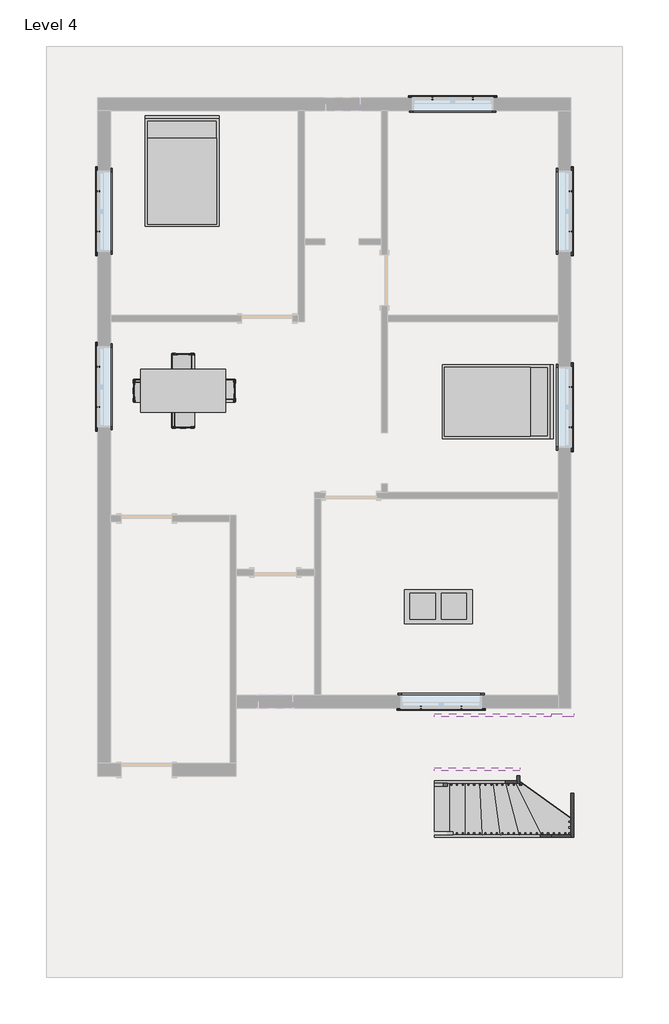
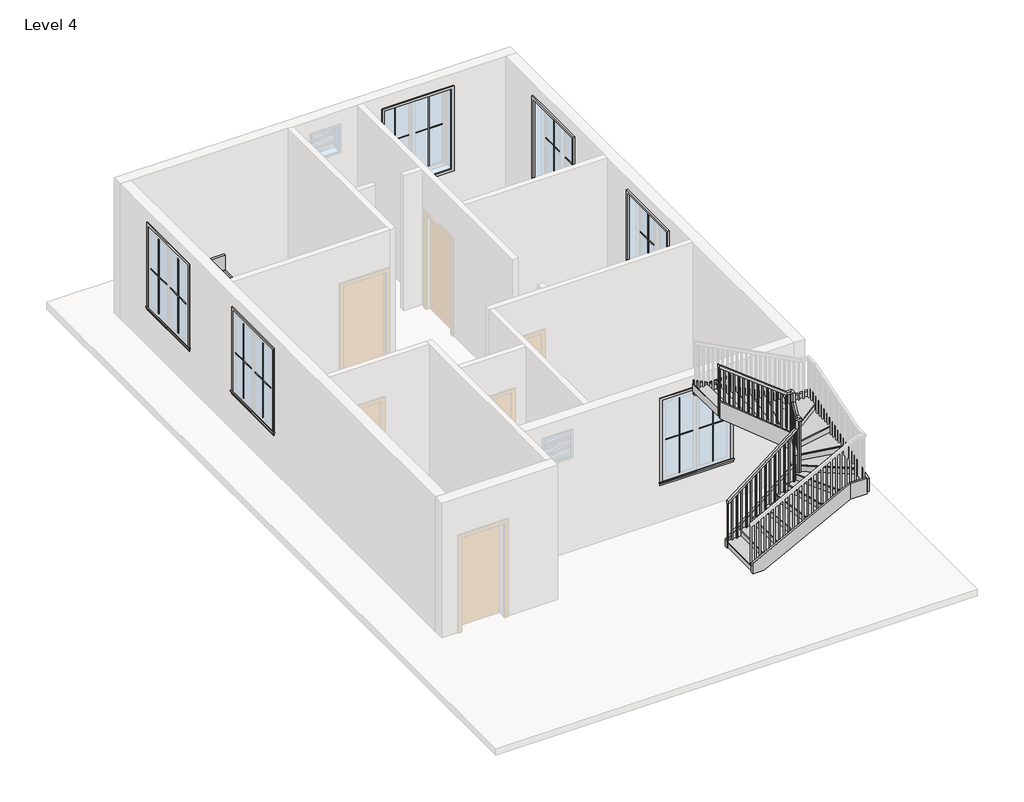
# One storey, part 3 of 3: 25 proxies, 8 members, 3 furniture elements, 1 railing, 1 stair flight.
"""IFC4 building model written with IfcOpenShell, lengths in millimetres."""

from ifc_helpers import new_model, si_unit, frame, origin, place, context, project, spatial, polyline, outline, extrude, faceted_brep, transform, mapped, element, save
from components import muntin_pattern_2x2_muntin_pattern_2x2_bff912c5, muntin_pattern_2x2_muntin_pattern_2x2_c2194282, trim_window_exterior_flat_with_sill_e04b3088, trim_window_interior_flat_picture_frame_2a7685fe, coffee_table_with_brass_mullions_11320_coffee_table_with_5962bef7, bed_17739_bed_17739_15c61121, dining_table_w_chairs_11374_0cdfc61b, stair_flight_8f30da42

model = new_model("IFC4")

# Units and contexts
model_context = context("Model", 3, world=origin())
ifc_project = project(units=[si_unit("LENGTHUNIT", "METRE", prefix="MILLI")], contexts=[model_context])

# Site, building, storey
site = spatial("IfcSite", under=ifc_project)
building = spatial("IfcBuilding", under=site)
storey = spatial("IfcBuildingStorey", under=building, Name="Level 4", Elevation=6400.8)

# Proxies
placement = place(None, origin())
muntin_pattern_2x2_muntin_pattern_2x2_shape = muntin_pattern_2x2_muntin_pattern_2x2_bff912c5(model_context)
element("IfcBuildingElementProxy", 1, Name="Muntin Pattern_2x2 : Muntin Pattern_2x2", ObjectType="Muntin Pattern_2x2 : Muntin Pattern_2x2", at=placement, inside=storey, context=model_context, shape_type="MappedRepresentation", body=[
    mapped(muntin_pattern_2x2_muntin_pattern_2x2_shape, transform((2964.3605034, 427.8534591, 7385.05), x_axis=(0.0, -1.0, 0.0), y_axis=(1.0, 0.0, 0.0), z_axis=(0.0, 0.0, 1.0))),
])
element("IfcBuildingElementProxy", 2, Name="Muntin Pattern_2x2 : Muntin Pattern_2x2", ObjectType="Muntin Pattern_2x2 : Muntin Pattern_2x2", at=placement, inside=storey, context=model_context, shape_type="MappedRepresentation", body=[
    mapped(muntin_pattern_2x2_muntin_pattern_2x2_shape, transform((2964.3605034, 3923.5284591, 7385.05), x_axis=(0.0, -1.0, 0.0), y_axis=(1.0, 0.0, 0.0), z_axis=(0.0, 0.0, 1.0))),
])
element("IfcBuildingElementProxy", 3, Name="Muntin Pattern_2x2 : Muntin Pattern_2x2", ObjectType="Muntin Pattern_2x2 : Muntin Pattern_2x2", at=placement, inside=storey, context=model_context, shape_type="MappedRepresentation", body=[
    mapped(muntin_pattern_2x2_muntin_pattern_2x2_shape, transform((498.9730034, 5582.4659591, 7385.05), x_axis=(1.0, 0.0, 0.0), y_axis=(0.0, 1.0, 0.0), z_axis=(0.0, 0.0, 1.0))),
])
element("IfcBuildingElementProxy", 4, Name="Muntin Pattern_2x2 : Muntin Pattern_2x2", ObjectType="Muntin Pattern_2x2 : Muntin Pattern_2x2", at=placement, inside=storey, context=model_context, shape_type="MappedRepresentation", body=[
    mapped(muntin_pattern_2x2_muntin_pattern_2x2_shape, transform((-5474.7894966, 3202.8034591, 7385.05), x_axis=(0.0, 1.0, 0.0), y_axis=(-1.0, 0.0, 0.0), z_axis=(0.0, 0.0, 1.0))),
])
element("IfcBuildingElementProxy", 5, Name="Muntin Pattern_2x2 : Muntin Pattern_2x2", ObjectType="Muntin Pattern_2x2 : Muntin Pattern_2x2", at=placement, inside=storey, context=model_context, shape_type="MappedRepresentation", body=[
    mapped(muntin_pattern_2x2_muntin_pattern_2x2_shape, transform((-5474.7894966, 69.0784591, 7385.05), x_axis=(0.0, 1.0, 0.0), y_axis=(-1.0, 0.0, 0.0), z_axis=(0.0, 0.0, 1.0))),
])
element("IfcBuildingElementProxy", 6, Name="Muntin Pattern_2x2 : Muntin Pattern_2x2", ObjectType="Muntin Pattern_2x2 : Muntin Pattern_2x2", at=placement, inside=storey, context=model_context, shape_type="MappedRepresentation", body=[
    mapped(muntin_pattern_2x2_muntin_pattern_2x2_shape, transform((1013.3230034, -5295.0840409, 7385.05), x_axis=(-1.0, 0.0, 0.0), y_axis=(0.0, -1.0, 0.0), z_axis=(0.0, 0.0, 1.0))),
])
muntin_pattern_2x2_muntin_pattern_2x2_2_shape = muntin_pattern_2x2_muntin_pattern_2x2_c2194282(model_context)
element("IfcBuildingElementProxy", 7, Name="Muntin Pattern_2x2 : Muntin Pattern_2x2", ObjectType="Muntin Pattern_2x2 : Muntin Pattern_2x2", at=placement, inside=storey, context=model_context, shape_type="MappedRepresentation", body=[
    mapped(muntin_pattern_2x2_muntin_pattern_2x2_2_shape, transform((2964.3605034, -292.8715409, 7385.05), x_axis=(0.0, 1.0, 0.0), y_axis=(-1.0, 0.0, 0.0), z_axis=(0.0, 0.0, 1.0))),
])
element("IfcBuildingElementProxy", 8, Name="Muntin Pattern_2x2 : Muntin Pattern_2x2", ObjectType="Muntin Pattern_2x2 : Muntin Pattern_2x2", at=placement, inside=storey, context=model_context, shape_type="MappedRepresentation", body=[
    mapped(muntin_pattern_2x2_muntin_pattern_2x2_2_shape, transform((2964.3605034, 3202.8034591, 7385.05), x_axis=(0.0, 1.0, 0.0), y_axis=(-1.0, 0.0, 0.0), z_axis=(0.0, 0.0, 1.0))),
])
element("IfcBuildingElementProxy", 9, Name="Muntin Pattern_2x2 : Muntin Pattern_2x2", ObjectType="Muntin Pattern_2x2 : Muntin Pattern_2x2", at=placement, inside=storey, context=model_context, shape_type="MappedRepresentation", body=[
    mapped(muntin_pattern_2x2_muntin_pattern_2x2_2_shape, transform((1219.6980034, 5582.4659591, 7385.05), x_axis=(-1.0, 0.0, 0.0), y_axis=(0.0, -1.0, 0.0), z_axis=(0.0, 0.0, 1.0))),
])
element("IfcBuildingElementProxy", 10, Name="Muntin Pattern_2x2 : Muntin Pattern_2x2", ObjectType="Muntin Pattern_2x2 : Muntin Pattern_2x2", at=placement, inside=storey, context=model_context, shape_type="MappedRepresentation", body=[
    mapped(muntin_pattern_2x2_muntin_pattern_2x2_2_shape, transform((-5474.7894966, 3923.5284591, 7385.05), x_axis=(0.0, -1.0, 0.0), y_axis=(1.0, 0.0, 0.0), z_axis=(0.0, 0.0, 1.0))),
])
element("IfcBuildingElementProxy", 11, Name="Muntin Pattern_2x2 : Muntin Pattern_2x2", ObjectType="Muntin Pattern_2x2 : Muntin Pattern_2x2", at=placement, inside=storey, context=model_context, shape_type="MappedRepresentation", body=[
    mapped(muntin_pattern_2x2_muntin_pattern_2x2_2_shape, transform((-5474.7894966, 789.8034591, 7385.05), x_axis=(0.0, -1.0, 0.0), y_axis=(1.0, 0.0, 0.0), z_axis=(0.0, 0.0, 1.0))),
])
element("IfcBuildingElementProxy", 12, Name="Muntin Pattern_2x2 : Muntin Pattern_2x2", ObjectType="Muntin Pattern_2x2 : Muntin Pattern_2x2", at=placement, inside=storey, context=model_context, shape_type="MappedRepresentation", body=[
    mapped(muntin_pattern_2x2_muntin_pattern_2x2_2_shape, transform((292.5980034, -5295.0840409, 7385.05), x_axis=(1.0, 0.0, 0.0), y_axis=(0.0, 1.0, 0.0), z_axis=(0.0, 0.0, 1.0))),
])
trim_window_exterior_flat_with_sill_shape = trim_window_exterior_flat_with_sill_e04b3088(model_context)
element("IfcBuildingElementProxy", 13, Name="Trim-Window-Exterior-Flat : with Sill", ObjectType="Trim-Window-Exterior-Flat : with Sill", at=placement, inside=storey, context=model_context, shape_type="MappedRepresentation", body=[
    mapped(trim_window_exterior_flat_with_sill_shape, transform((2973.8855034, 67.4909591, 9144.0), x_axis=(0.0, 1.0, 0.0), y_axis=(0.0, 0.0, 1.0), z_axis=(1.0, 0.0, 0.0))),
])
element("IfcBuildingElementProxy", 14, Name="Trim-Window-Exterior-Flat : with Sill", ObjectType="Trim-Window-Exterior-Flat : with Sill", at=placement, inside=storey, context=model_context, shape_type="MappedRepresentation", body=[
    mapped(trim_window_exterior_flat_with_sill_shape, transform((2973.8855034, 3563.1659591, 9144.0), x_axis=(0.0, 1.0, 0.0), y_axis=(0.0, 0.0, 1.0), z_axis=(1.0, 0.0, 0.0))),
])
element("IfcBuildingElementProxy", 15, Name="Trim-Window-Exterior-Flat : with Sill", ObjectType="Trim-Window-Exterior-Flat : with Sill", at=placement, inside=storey, context=model_context, shape_type="MappedRepresentation", body=[
    mapped(trim_window_exterior_flat_with_sill_shape, transform((859.3355034, 5591.9909591, 9144.0), x_axis=(-1.0, 0.0, 0.0), y_axis=(0.0, 0.0, 1.0), z_axis=(0.0, 1.0, 0.0))),
])
element("IfcBuildingElementProxy", 16, Name="Trim-Window-Exterior-Flat : with Sill", ObjectType="Trim-Window-Exterior-Flat : with Sill", at=placement, inside=storey, context=model_context, shape_type="MappedRepresentation", body=[
    mapped(trim_window_exterior_flat_with_sill_shape, transform((-5484.3144966, 3563.1659591, 9144.0), x_axis=(0.0, -1.0, 0.0), y_axis=(0.0, 0.0, 1.0), z_axis=(-1.0, 0.0, 0.0))),
])
element("IfcBuildingElementProxy", 17, Name="Trim-Window-Exterior-Flat : with Sill", ObjectType="Trim-Window-Exterior-Flat : with Sill", at=placement, inside=storey, context=model_context, shape_type="MappedRepresentation", body=[
    mapped(trim_window_exterior_flat_with_sill_shape, transform((-5484.3144966, 429.4409591, 9144.0), x_axis=(0.0, -1.0, 0.0), y_axis=(0.0, 0.0, 1.0), z_axis=(-1.0, 0.0, 0.0))),
])
element("IfcBuildingElementProxy", 18, Name="Trim-Window-Exterior-Flat : with Sill", ObjectType="Trim-Window-Exterior-Flat : with Sill", at=placement, inside=storey, context=model_context, shape_type="MappedRepresentation", body=[
    mapped(trim_window_exterior_flat_with_sill_shape, transform((652.9605034, -5304.6090409, 9144.0), x_axis=(1.0, 0.0, 0.0), y_axis=(0.0, 0.0, 1.0), z_axis=(0.0, -1.0, 0.0))),
])
trim_window_interior_flat_picture_frame_shape = trim_window_interior_flat_picture_frame_2a7685fe(model_context)
element("IfcBuildingElementProxy", 19, Name="Trim-Window-Interior-Flat : Picture Frame", ObjectType="Trim-Window-Interior-Flat : Picture Frame", at=placement, inside=storey, context=model_context, shape_type="MappedRepresentation", body=[
    mapped(trim_window_interior_flat_picture_frame_shape, transform((2745.2855034, 67.4909591, 9144.0), x_axis=(0.0, -1.0, 0.0), y_axis=(0.0, 0.0, 1.0), z_axis=(-1.0, 0.0, 0.0))),
])
element("IfcBuildingElementProxy", 20, Name="Trim-Window-Interior-Flat : Picture Frame", ObjectType="Trim-Window-Interior-Flat : Picture Frame", at=placement, inside=storey, context=model_context, shape_type="MappedRepresentation", body=[
    mapped(trim_window_interior_flat_picture_frame_shape, transform((2745.2855034, 3563.1659591, 9144.0), x_axis=(0.0, -1.0, 0.0), y_axis=(0.0, 0.0, 1.0), z_axis=(-1.0, 0.0, 0.0))),
])
element("IfcBuildingElementProxy", 21, Name="Trim-Window-Interior-Flat : Picture Frame", ObjectType="Trim-Window-Interior-Flat : Picture Frame", at=placement, inside=storey, context=model_context, shape_type="MappedRepresentation", body=[
    mapped(trim_window_interior_flat_picture_frame_shape, transform((859.3355034, 5363.3909591, 9144.0), x_axis=(1.0, 0.0, 0.0), y_axis=(0.0, 0.0, 1.0), z_axis=(0.0, -1.0, 0.0))),
])
element("IfcBuildingElementProxy", 22, Name="Trim-Window-Interior-Flat : Picture Frame", ObjectType="Trim-Window-Interior-Flat : Picture Frame", at=placement, inside=storey, context=model_context, shape_type="MappedRepresentation", body=[
    mapped(trim_window_interior_flat_picture_frame_shape, transform((-5255.7144966, 3563.1659591, 9144.0), x_axis=(0.0, 1.0, 0.0), y_axis=(0.0, 0.0, 1.0), z_axis=(1.0, 0.0, 0.0))),
])
element("IfcBuildingElementProxy", 23, Name="Trim-Window-Interior-Flat : Picture Frame", ObjectType="Trim-Window-Interior-Flat : Picture Frame", at=placement, inside=storey, context=model_context, shape_type="MappedRepresentation", body=[
    mapped(trim_window_interior_flat_picture_frame_shape, transform((-5255.7144966, 429.4409591, 9144.0), x_axis=(0.0, 1.0, 0.0), y_axis=(0.0, 0.0, 1.0), z_axis=(1.0, 0.0, 0.0))),
])
element("IfcBuildingElementProxy", 24, Name="Trim-Window-Interior-Flat : Picture Frame", ObjectType="Trim-Window-Interior-Flat : Picture Frame", at=placement, inside=storey, context=model_context, shape_type="MappedRepresentation", body=[
    mapped(trim_window_interior_flat_picture_frame_shape, transform((652.9605034, -5076.0090409, 9144.0), x_axis=(-1.0, 0.0, 0.0), y_axis=(0.0, 0.0, 1.0), z_axis=(0.0, 1.0, 0.0))),
])
coffee_table_with_brass_mullions_11320_coffee_table_with_shape = coffee_table_with_brass_mullions_11320_coffee_table_with_5962bef7(model_context)
element("IfcBuildingElementProxy", 25, Name="coffee_table_with_brass_mullions_11320 : coffee_table_with_brass_mullions_11320", ObjectType="coffee_table_with_brass_mullions_11320 : coffee_table_with_brass_mullions_11320", at=placement, inside=storey, context=model_context, shape_type="MappedRepresentation", body=[
    mapped(coffee_table_with_brass_mullions_11320_coffee_table_with_shape, transform((1240.0943553, -3926.0808329, 6400.8), x_axis=(1.0, 0.0, 0.0), y_axis=(0.0, 1.0, 0.0), z_axis=(0.0, 0.0, 1.0))),
])

# Furniture
bed_17739_bed_17739_shape = bed_17739_bed_17739_15c61121(model_context)
element("IfcFurniture", 26, ObjectType="Bed_17739 : Bed_17739", at=placement, inside=storey, context=model_context, shape_type="MappedRepresentation", body=[
    mapped(bed_17739_bed_17739_shape, transform((-3979.3644966, 4258.4909591, 6400.8), x_axis=(1.0, 0.0, 0.0), y_axis=(0.0, 1.0, 0.0), z_axis=(0.0, 0.0, 1.0))),
])
element("IfcFurniture", 27, ObjectType="Bed_17739 : Bed_17739", at=placement, inside=storey, context=model_context, shape_type="MappedRepresentation", body=[
    mapped(bed_17739_bed_17739_shape, transform((1640.3855034, 162.7409591, 6400.8), x_axis=(0.0, -1.0, 0.0), y_axis=(1.0, 0.0, 0.0), z_axis=(0.0, 0.0, 1.0))),
])
dining_table_w_chairs_11374_shape = dining_table_w_chairs_11374_0cdfc61b(model_context)
element("IfcFurniture", 28, ObjectType="Dining_Table_w_Chairs_11374", at=placement, inside=storey, context=model_context, shape_type="MappedRepresentation", body=[
    mapped(dining_table_w_chairs_11374_shape, transform((-3975.2132663, 265.1952874, 6400.8), x_axis=(1.0, 0.0, 0.0), y_axis=(0.0, 1.0, 0.0), z_axis=(0.0, 0.0, 1.0))),
])

# Members
element("IfcMember", 29, ObjectType="Stringer - 2\" Width", at=placement, inside=storey, context=model_context, shape_type="SweptSolid", body=[
    extrude(outline(polyline([(6576.9764461, 531.7538115), (6400.8, 531.7538115), (6400.8, 798.0154561), (7387.9410923, 2008.6855034), (7781.218648, 2008.6855034), (6576.9764461, 531.7538115)])), frame((0.0, -6650.8090409, 0.0), z_axis=(0.0, 1.0, 0.0), x_axis=(0.0, 0.0, 1.0)), (0.0, 0.0, 1.0), 50.8),
])
element("IfcMember", 30, ObjectType="Stringer - 2\" Width", at=placement, inside=storey, context=model_context, shape_type="SweptSolid", body=[
    extrude(outline(polyline([(-6650.8090409, 7429.3617647), (-6650.8090409, 7974.0682978), (-6444.1719234, 8326.9409689), (-6422.2090409, 8326.9409689), (-6422.2090409, 7761.265107), (-6616.5668235, 7429.3617647), (-6650.8090409, 7429.3617647)])), frame((2008.6855034, 0.0, 0.0), z_axis=(1.0, 0.0, 0.0), x_axis=(0.0, 1.0, 0.0)), (0.0, 0.0, 1.0), 50.8),
])
element("IfcMember", 31, ObjectType="Stringer - 2\" Width", at=placement, inside=storey, context=model_context, shape_type="SweptSolid", body=[
    extrude(outline(polyline([(7933.6634131, 2059.4855034), (8326.9409689, 2059.4855034), (9572.6038432, 531.7538115), (9179.3262875, 531.7538115), (7933.6634131, 2059.4855034)])), frame((0.0, -6422.2090409, 0.0), z_axis=(0.0, 1.0, 0.0), x_axis=(0.0, 0.0, 1.0)), (0.0, 0.0, 1.0), 50.8),
])
element("IfcMember", 32, ObjectType="Stringer - 2\" Width", at=placement, inside=storey, context=model_context, shape_type="SweptSolid", body=[
    extrude(outline(polyline([(6630.439954, 531.7538115), (6400.8, 531.7538115), (6400.8, 751.5161291), (7363.300629, 2619.1710032), (7706.1956453, 2619.1710032), (6630.439954, 531.7538115)])), frame((0.0, -7616.0090409, 0.0), z_axis=(0.0, 1.0, 0.0), x_axis=(0.0, 0.0, 1.0)), (0.0, 0.0, 1.0), 50.8),
])
element("IfcMember", 33, ObjectType="Stringer - 2\" Width", at=placement, inside=storey, context=model_context, shape_type="SweptSolid", body=[
    extrude(outline(polyline([(2619.1710032, -7616.0090409), (2619.1710032, -7565.2090409), (2973.8855034, -7565.2090409), (2973.8855034, -7616.0090409), (2619.1710032, -7616.0090409)])), frame((0.0, 0.0, 7363.300629), z_axis=(0.0, 0.0, 1.0), x_axis=(1.0, 0.0, 0.0)), (0.0, 0.0, 1.0), 342.8950162),
])
element("IfcMember", 34, ObjectType="Stringer - 2\" Width", at=placement, inside=storey, context=model_context, shape_type="SweptSolid", body=[
    extrude(outline(polyline([(-7616.0090409, 7401.3956453), (-7616.0090409, 7689.8952212), (-5493.9891581, 8370.7972697), (-5457.0090409, 8370.7972697), (-5457.0090409, 8039.7682298), (-7446.4865579, 7401.3956453), (-7616.0090409, 7401.3956453)])), frame((2973.8855034, 0.0, 0.0), z_axis=(1.0, 0.0, 0.0), x_axis=(0.0, 1.0, 0.0)), (0.0, 0.0, 1.0), 50.8),
])
element("IfcMember", 35, ObjectType="Stringer - 2\" Width", at=placement, inside=storey, context=model_context, shape_type="SweptSolid", body=[
    extrude(outline(polyline([(3024.6855034, -5406.2090409), (3024.6855034, -5457.0090409), (2619.1710032, -5457.0090409), (2619.1710032, -5406.2090409), (3024.6855034, -5406.2090409)])), frame((0.0, 0.0, 8050.6904473), z_axis=(0.0, 0.0, 1.0), x_axis=(1.0, 0.0, 0.0)), (0.0, 0.0, 1.0), 320.1068224),
])
element("IfcMember", 36, ObjectType="Stringer - 2\" Width", at=placement, inside=storey, context=model_context, shape_type="SweptSolid", body=[
    extrude(outline(polyline([(8050.6904473, 2619.1710032), (8370.7972697, 2619.1710032), (9446.5529609, 531.7538115), (9126.4461385, 531.7538115), (8050.6904473, 2619.1710032)])), frame((0.0, -5457.0090409, 0.0), z_axis=(0.0, 1.0, 0.0), x_axis=(0.0, 0.0, 1.0)), (0.0, 0.0, 1.0), 50.8),
])

# Railing
element("IfcRailing", 37, ObjectType="Handrail - Rectangular", at=placement, inside=storey, context=model_context, shape_type="SolidModel", body=[
    faceted_brep([(531.7538115, -6650.8090409, 7484.5333333), (531.7538115, -6650.8090409, 7420.2000346), (531.7538115, -6701.6090409, 7420.2000346), (531.7538115, -6701.6090409, 7484.5333333), (1983.2855034, -6650.8090409, 8612.4191036), (2034.0855034, -6650.8090409, 8587.5590024), (2034.0855034, -6701.6090409, 8587.5590024), (1983.2855034, -6701.6090409, 8612.4191036), (2059.4855034, -6545.487707, 8764.6281882), (2059.4855034, -6574.6090409, 8815.4281882), (2059.4855034, -6447.6090409, 9032.3051451), (2059.4855034, -6396.8090409, 9018.5256424), (2110.2855034, -6545.487707, 8764.6281882), (2110.2855034, -6396.8090409, 9018.5256424), (2110.2855034, -6574.6090409, 8815.4281882), (2110.2855034, -6447.6090409, 9032.3051451), (531.7538115, -6371.4090409, 10363.2), (531.7538115, -6320.6090409, 10363.2), (531.7538115, -6320.6090409, 10298.8667013), (531.7538115, -6371.4090409, 10298.8667013), (1965.8688354, -6371.4090409, 9184.5142297), (1983.2855034, -6371.4090409, 9235.3142297), (1965.8688354, -6320.6090409, 9184.5142297), (1983.2855034, -6320.6090409, 9235.3142297), (1983.2855034, -6650.8090409, 8815.4281882), (2034.0855034, -6650.8090409, 8764.6281882), (2034.0855034, -6701.6090409, 8764.6281882), (1983.2855034, -6701.6090409, 8815.4281882), (2059.4855034, -6650.8090409, 8815.4281882), (2059.4855034, -6650.8090409, 8764.6281882), (2110.2855034, -6701.6090409, 8764.6281882), (2110.2855034, -6701.6090409, 8815.4281882), (2059.4855034, -6447.6090409, 9235.3142297), (2059.4855034, -6396.8090409, 9184.5142297), (2110.2855034, -6396.8090409, 9184.5142297), (2110.2855034, -6447.6090409, 9235.3142297), (2059.4855034, -6371.4090409, 9235.3142297), (2059.4855034, -6371.4090409, 9184.5142297), (2110.2855034, -6320.6090409, 9184.5142297), (2110.2855034, -6320.6090409, 9235.3142297)], [[[0, 1, 2, 3]], [[1, 0, 4, 5]], [[2, 1, 5, 6]], [[3, 2, 6, 7]], [[0, 3, 7, 4]], [[8, 9, 10, 11]], [[12, 8, 11, 13]], [[14, 12, 13, 15]], [[9, 14, 15, 10]], [[16, 17, 18, 19]], [[20, 21, 16, 19]], [[22, 20, 19, 18]], [[23, 22, 18, 17]], [[21, 23, 17, 16]], [[5, 4, 24, 25]], [[6, 5, 25, 26]], [[7, 6, 26, 27]], [[4, 7, 27, 24]], [[25, 24, 28, 29]], [[26, 25, 29, 30]], [[27, 26, 30, 31]], [[24, 27, 31, 28]], [[29, 28, 9, 8]], [[30, 29, 8, 12]], [[31, 30, 12, 14]], [[28, 31, 14, 9]], [[11, 10, 32, 33]], [[13, 11, 33, 34]], [[15, 13, 34, 35]], [[10, 15, 35, 32]], [[33, 32, 36, 37]], [[34, 33, 37, 38]], [[35, 34, 38, 39]], [[32, 35, 39, 36]], [[37, 36, 21, 20]], [[38, 37, 20, 22]], [[39, 38, 22, 23]], [[36, 39, 23, 21]]]),
    extrude(outline(polyline([(10283.6316852, 551.3605034), (9279.4666667, 551.3605034), (9279.4666667, 570.4105034), (10268.8292361, 570.4105034), (10283.6316852, 551.3605034)])), frame((0.0, -6355.5340409, 0.0), z_axis=(0.0, 1.0, 0.0), x_axis=(0.0, 0.0, 1.0)), (0.0, 0.0, 1.0), 19.05),
    extrude(outline(polyline([(10204.6852902, 652.9605034), (9279.4666667, 652.9605034), (9279.4666667, 672.0105034), (10189.8828411, 672.0105034), (10204.6852902, 652.9605034)])), frame((0.0, -6355.5340409, 0.0), z_axis=(0.0, 1.0, 0.0), x_axis=(0.0, 0.0, 1.0)), (0.0, 0.0, 1.0), 19.05),
    extrude(outline(polyline([(10125.7388952, 754.5605034), (9279.4666667, 754.5605034), (9279.4666667, 773.6105034), (10110.9364462, 773.6105034), (10125.7388952, 754.5605034)])), frame((0.0, -6355.5340409, 0.0), z_axis=(0.0, 1.0, 0.0), x_axis=(0.0, 0.0, 1.0)), (0.0, 0.0, 1.0), 19.05),
    extrude(outline(polyline([(10046.7925003, 856.1605034), (9110.1333333, 856.1605034), (9110.1333333, 875.2105034), (10031.9900512, 875.2105034), (10046.7925003, 856.1605034)])), frame((0.0, -6355.5340409, 0.0), z_axis=(0.0, 1.0, 0.0), x_axis=(0.0, 0.0, 1.0)), (0.0, 0.0, 1.0), 19.05),
    extrude(outline(polyline([(9967.8461053, 957.7605034), (9110.1333333, 957.7605034), (9110.1333333, 976.8105034), (9953.0436562, 976.8105034), (9967.8461053, 957.7605034)])), frame((0.0, -6355.5340409, 0.0), z_axis=(0.0, 1.0, 0.0), x_axis=(0.0, 0.0, 1.0)), (0.0, 0.0, 1.0), 19.05),
    extrude(outline(polyline([(9888.8997103, 1059.3605034), (9110.1333333, 1059.3605034), (9110.1333333, 1078.4105034), (9874.0972613, 1078.4105034), (9888.8997103, 1059.3605034)])), frame((0.0, -6355.5340409, 0.0), z_axis=(0.0, 1.0, 0.0), x_axis=(0.0, 0.0, 1.0)), (0.0, 0.0, 1.0), 19.05),
    extrude(outline(polyline([(9809.9533154, 1160.9605034), (8940.8, 1160.9605034), (8940.8, 1180.0105034), (9795.1508663, 1180.0105034), (9809.9533154, 1160.9605034)])), frame((0.0, -6355.5340409, 0.0), z_axis=(0.0, 1.0, 0.0), x_axis=(0.0, 0.0, 1.0)), (0.0, 0.0, 1.0), 19.05),
    extrude(outline(polyline([(9731.0069204, 1262.5605034), (8940.8, 1262.5605034), (8940.8, 1281.6105034), (9716.2044713, 1281.6105034), (9731.0069204, 1262.5605034)])), frame((0.0, -6355.5340409, 0.0), z_axis=(0.0, 1.0, 0.0), x_axis=(0.0, 0.0, 1.0)), (0.0, 0.0, 1.0), 19.05),
    extrude(outline(polyline([(9652.0605254, 1364.1605034), (8771.4666667, 1364.1605034), (8771.4666667, 1383.2105034), (9637.2580764, 1383.2105034), (9652.0605254, 1364.1605034)])), frame((0.0, -6355.5340409, 0.0), z_axis=(0.0, 1.0, 0.0), x_axis=(0.0, 0.0, 1.0)), (0.0, 0.0, 1.0), 19.05),
    extrude(outline(polyline([(9573.1141304, 1465.7605034), (8771.4666667, 1465.7605034), (8771.4666667, 1484.8105034), (9558.3116814, 1484.8105034), (9573.1141304, 1465.7605034)])), frame((0.0, -6355.5340409, 0.0), z_axis=(0.0, 1.0, 0.0), x_axis=(0.0, 0.0, 1.0)), (0.0, 0.0, 1.0), 19.05),
    extrude(outline(polyline([(9494.1677355, 1567.3605034), (8771.4666667, 1567.3605034), (8771.4666667, 1586.4105034), (9479.3652864, 1586.4105034), (9494.1677355, 1567.3605034)])), frame((0.0, -6355.5340409, 0.0), z_axis=(0.0, 1.0, 0.0), x_axis=(0.0, 0.0, 1.0)), (0.0, 0.0, 1.0), 19.05),
    extrude(outline(polyline([(9415.2213405, 1668.9605034), (8602.1333333, 1668.9605034), (8602.1333333, 1688.0105034), (9400.4188914, 1688.0105034), (9415.2213405, 1668.9605034)])), frame((0.0, -6355.5340409, 0.0), z_axis=(0.0, 1.0, 0.0), x_axis=(0.0, 0.0, 1.0)), (0.0, 0.0, 1.0), 19.05),
    extrude(outline(polyline([(9336.2749455, 1770.5605034), (8602.1333333, 1770.5605034), (8602.1333333, 1789.6105034), (9321.4724965, 1789.6105034), (9336.2749455, 1770.5605034)])), frame((0.0, -6355.5340409, 0.0), z_axis=(0.0, 1.0, 0.0), x_axis=(0.0, 0.0, 1.0)), (0.0, 0.0, 1.0), 19.05),
    extrude(outline(polyline([(9257.3285506, 1872.1605034), (8432.8, 1872.1605034), (8432.8, 1891.2105034), (9242.5261015, 1891.2105034), (9257.3285506, 1872.1605034)])), frame((0.0, -6355.5340409, 0.0), z_axis=(0.0, 1.0, 0.0), x_axis=(0.0, 0.0, 1.0)), (0.0, 0.0, 1.0), 19.05),
    extrude(outline(polyline([(9178.3821556, 1973.7605034), (8432.8, 1973.7605034), (8432.8, 1992.8105034), (9163.5797065, 1992.8105034), (9178.3821556, 1973.7605034)])), frame((0.0, -6355.5340409, 0.0), z_axis=(0.0, 1.0, 0.0), x_axis=(0.0, 0.0, 1.0)), (0.0, 0.0, 1.0), 19.05),
    extrude(outline(polyline([(2075.3605034, -6380.9340409), (2075.3605034, -6361.8840409), (2094.4105034, -6361.8840409), (2094.4105034, -6380.9340409), (2075.3605034, -6380.9340409)])), frame((0.0, 0.0, 8094.1333333), z_axis=(0.0, 0.0, 1.0), x_axis=(1.0, 0.0, 0.0)), (0.0, 0.0, 1.0), 1090.3808964),
    extrude(outline(polyline([(-6463.4840409, 8904.66524), (-6463.4840409, 7924.8), (-6482.5340409, 7924.8), (-6482.5340409, 8872.1336964), (-6463.4840409, 8904.66524)])), frame((2075.3605034, 0.0, 0.0), z_axis=(1.0, 0.0, 0.0), x_axis=(0.0, 1.0, 0.0)), (0.0, 0.0, 1.0), 19.05),
    extrude(outline(polyline([(-6565.0840409, 8731.1636744), (-6565.0840409, 7755.4666667), (-6584.1340409, 7755.4666667), (-6584.1340409, 8698.6321309), (-6565.0840409, 8731.1636744)])), frame((2075.3605034, 0.0, 0.0), z_axis=(1.0, 0.0, 0.0), x_axis=(0.0, 1.0, 0.0)), (0.0, 0.0, 1.0), 19.05),
    extrude(outline(polyline([(2046.2288115, -6666.6840409), (2065.2788115, -6666.6840409), (2065.2788115, -6685.7340409), (2046.2288115, -6685.7340409), (2046.2288115, -6666.6840409)])), frame((0.0, 0.0, 7586.1333333), z_axis=(0.0, 0.0, 1.0), x_axis=(1.0, 0.0, 0.0)), (0.0, 0.0, 1.0), 1178.4948549),
    extrude(outline(polyline([(8518.0483397, 1944.6288115), (7416.8, 1944.6288115), (7416.8, 1963.6788115), (8532.8507888, 1963.6788115), (8518.0483397, 1944.6288115)])), frame((0.0, -6685.7340409, 0.0), z_axis=(0.0, 1.0, 0.0), x_axis=(0.0, 0.0, 1.0)), (0.0, 0.0, 1.0), 19.05),
    extrude(outline(polyline([(8439.1019447, 1843.0288115), (7416.8, 1843.0288115), (7416.8, 1862.0788115), (8453.9043938, 1862.0788115), (8439.1019447, 1843.0288115)])), frame((0.0, -6685.7340409, 0.0), z_axis=(0.0, 1.0, 0.0), x_axis=(0.0, 0.0, 1.0)), (0.0, 0.0, 1.0), 19.05),
    extrude(outline(polyline([(8360.1555498, 1741.4288115), (7247.4666667, 1741.4288115), (7247.4666667, 1760.4788115), (8374.9579988, 1760.4788115), (8360.1555498, 1741.4288115)])), frame((0.0, -6685.7340409, 0.0), z_axis=(0.0, 1.0, 0.0), x_axis=(0.0, 0.0, 1.0)), (0.0, 0.0, 1.0), 19.05),
    extrude(outline(polyline([(8281.2091548, 1639.8288115), (7247.4666667, 1639.8288115), (7247.4666667, 1658.8788115), (8296.0116039, 1658.8788115), (8281.2091548, 1639.8288115)])), frame((0.0, -6685.7340409, 0.0), z_axis=(0.0, 1.0, 0.0), x_axis=(0.0, 0.0, 1.0)), (0.0, 0.0, 1.0), 19.05),
    extrude(outline(polyline([(8202.2627598, 1538.2288115), (7078.1333333, 1538.2288115), (7078.1333333, 1557.2788115), (8217.0652089, 1557.2788115), (8202.2627598, 1538.2288115)])), frame((0.0, -6685.7340409, 0.0), z_axis=(0.0, 1.0, 0.0), x_axis=(0.0, 0.0, 1.0)), (0.0, 0.0, 1.0), 19.05),
    extrude(outline(polyline([(8123.3163649, 1436.6288115), (7078.1333333, 1436.6288115), (7078.1333333, 1455.6788115), (8138.1188139, 1455.6788115), (8123.3163649, 1436.6288115)])), frame((0.0, -6685.7340409, 0.0), z_axis=(0.0, 1.0, 0.0), x_axis=(0.0, 0.0, 1.0)), (0.0, 0.0, 1.0), 19.05),
    extrude(outline(polyline([(8044.3699699, 1335.0288115), (6908.8, 1335.0288115), (6908.8, 1354.0788115), (8059.1724189, 1354.0788115), (8044.3699699, 1335.0288115)])), frame((0.0, -6685.7340409, 0.0), z_axis=(0.0, 1.0, 0.0), x_axis=(0.0, 0.0, 1.0)), (0.0, 0.0, 1.0), 19.05),
    extrude(outline(polyline([(7965.4235749, 1233.4288115), (6908.8, 1233.4288115), (6908.8, 1252.4788115), (7980.226024, 1252.4788115), (7965.4235749, 1233.4288115)])), frame((0.0, -6685.7340409, 0.0), z_axis=(0.0, 1.0, 0.0), x_axis=(0.0, 0.0, 1.0)), (0.0, 0.0, 1.0), 19.05),
    extrude(outline(polyline([(7886.4771799, 1131.8288115), (6908.8, 1131.8288115), (6908.8, 1150.8788115), (7901.279629, 1150.8788115), (7886.4771799, 1131.8288115)])), frame((0.0, -6685.7340409, 0.0), z_axis=(0.0, 1.0, 0.0), x_axis=(0.0, 0.0, 1.0)), (0.0, 0.0, 1.0), 19.05),
    extrude(outline(polyline([(7807.530785, 1030.2288115), (6739.4666667, 1030.2288115), (6739.4666667, 1049.2788115), (7822.333234, 1049.2788115), (7807.530785, 1030.2288115)])), frame((0.0, -6685.7340409, 0.0), z_axis=(0.0, 1.0, 0.0), x_axis=(0.0, 0.0, 1.0)), (0.0, 0.0, 1.0), 19.05),
    extrude(outline(polyline([(7728.58439, 928.6288115), (6739.4666667, 928.6288115), (6739.4666667, 947.6788115), (7743.3868391, 947.6788115), (7728.58439, 928.6288115)])), frame((0.0, -6685.7340409, 0.0), z_axis=(0.0, 1.0, 0.0), x_axis=(0.0, 0.0, 1.0)), (0.0, 0.0, 1.0), 19.05),
    extrude(outline(polyline([(7649.637995, 827.0288115), (6739.4666667, 827.0288115), (6739.4666667, 846.0788115), (7664.4404441, 846.0788115), (7649.637995, 827.0288115)])), frame((0.0, -6685.7340409, 0.0), z_axis=(0.0, 1.0, 0.0), x_axis=(0.0, 0.0, 1.0)), (0.0, 0.0, 1.0), 19.05),
    extrude(outline(polyline([(7570.6916001, 725.4288115), (6570.1333333, 725.4288115), (6570.1333333, 744.4788115), (7585.4940491, 744.4788115), (7570.6916001, 725.4288115)])), frame((0.0, -6685.7340409, 0.0), z_axis=(0.0, 1.0, 0.0), x_axis=(0.0, 0.0, 1.0)), (0.0, 0.0, 1.0), 19.05),
    extrude(outline(polyline([(7491.7452051, 623.8288115), (6570.1333333, 623.8288115), (6570.1333333, 642.8788115), (7506.5476541, 642.8788115), (7491.7452051, 623.8288115)])), frame((0.0, -6685.7340409, 0.0), z_axis=(0.0, 1.0, 0.0), x_axis=(0.0, 0.0, 1.0)), (0.0, 0.0, 1.0), 19.05),
    extrude(outline(polyline([(2075.3605034, -6355.5340409), (2075.3605034, -6336.4840409), (2094.4105034, -6336.4840409), (2094.4105034, -6355.5340409), (2075.3605034, -6355.5340409)])), frame((0.0, 0.0, 8263.4666667), z_axis=(0.0, 0.0, 1.0), x_axis=(1.0, 0.0, 0.0)), (0.0, 0.0, 1.0), 921.0475631),
    extrude(outline(polyline([(2075.3605034, -6666.6840409), (2094.4105034, -6666.6840409), (2094.4105034, -6685.7340409), (2075.3605034, -6685.7340409), (2075.3605034, -6666.6840409)])), frame((0.0, 0.0, 7586.1333333), z_axis=(0.0, 0.0, 1.0), x_axis=(1.0, 0.0, 0.0)), (0.0, 0.0, 1.0), 1178.4948549),
    extrude(outline(polyline([(10298.8667013, 531.7538115), (9279.4666667, 531.7538115), (9279.4666667, 550.8038115), (10284.0642523, 550.8038115), (10298.8667013, 531.7538115)])), frame((0.0, -6355.5340409, 0.0), z_axis=(0.0, 1.0, 0.0), x_axis=(0.0, 0.0, 1.0)), (0.0, 0.0, 1.0), 19.05),
    extrude(outline(polyline([(7420.2000346, 531.7538115), (6570.1333333, 531.7538115), (6570.1333333, 550.8038115), (7435.0024837, 550.8038115), (7420.2000346, 531.7538115)])), frame((0.0, -6685.7340409, 0.0), z_axis=(0.0, 1.0, 0.0), x_axis=(0.0, 0.0, 1.0)), (0.0, 0.0, 1.0), 19.05),
])

# Stair flight
stair_flight_shape = stair_flight_8f30da42(model_context)
element("IfcStairFlight", 38, ObjectType="2\" Tread 1\" Nosing 1/4\" Riser", at=placement, inside=storey, context=model_context, shape_type="MappedRepresentation", body=[
    mapped(stair_flight_shape, transform((0.0, 0.0, 0.0), x_axis=(1.0, 0.0, 0.0), y_axis=(0.0, 1.0, 0.0), z_axis=(0.0, 0.0, 1.0))),
])

save(model, "model.ifc")

# Revit data of these elements
# Type "Muntin Pattern_2x2 : Muntin Pattern_2x2"
#   Width [instance default] = 4' - 0"
#   Thickness = 0' - 0 1/2"
#   Height [instance default] = 4' - 0"
#   Distance = 0' - 0 3/4"
#   Interior Material [instance default] = none
#   Exterior Material [instance default] = none
#   Default Elevation = 0
# Type "Trim-Window-Exterior-Flat : with Sill"
#   Trim Width = 0' - 2 1/4"
#   Trim Thickness_Picture Frame = 0' - 1 1/4"
#   Trim Thickness_with Sill = 0' - 0 3/4"
#   Sill Thickness = 0' - 1 1/4"
#   Opening Width [instance default] = 2' - 0"
#   Opening Height [instance default] = 3' - 0"
#   Default Elevation = 4' - 0"
#   Sill = yes
#   Picture Frame = no
#   Trim Material [instance default] = none
# Type "Trim-Window-Interior-Flat : Picture Frame"
#   Trim Thickness_Picture Frame = 0' - 1 1/4"
#   Trim Width = 0' - 2 1/4"
#   Trim Thickness_with Sill = 0' - 0 3/4"
#   Sill Thickness = 0' - 1 1/4"
#   Opening Width [instance default] = 2' - 0"
#   Opening Height [instance default] = 3' - 0"
#   Default Elevation = 4' - 0"
#   Sill = no
#   Picture Frame = yes
#   Trim Material [instance default] = none
# Type "coffee_table_with_brass_mullions_11320 : coffee_table_with_brass_mullions_11320"
#   Default Elevation = 0
# Type "Bed_17739 : Bed_17739"
#   Default Elevation = 0
# Type "Dining_Table_w_Chairs_11374"
#   Default Elevation = 0
#   Assembly Code = ""
# Type "Handrail - Rectangular"
#   Assembly Code = "C2010400"
#   built-in parameter 1008612 = 0.0416667 (stored number, unit not read)
#   built-in parameter 1008611 = 0.0416667 (stored number, unit not read)
#   built-in parameter 1008609 = 0.333333 (stored number, unit not read)
#   built-in parameter 1008604 = 0.166667 (stored number, unit not read)
#   built-in parameter 1008603 = 0.166667 (stored number, unit not read)
#   Railing Height = 3' - 0"
#   built-in parameter 1008630 = 2
#   built-in parameter 1008610 = 2
#   built-in parameter 1008618 = Baluster - Square : 3/4"
# Elements 1, 2, 3, 4, 5, 6, 7, 8, 9, 10, 11, 12 (IfcBuildingElementProxy, "Muntin Pattern_2x2 : Muntin Pattern_2x2")
#   Width = 1' - 11 1/8"
#   Height = 5' - 6 1/2"
#   Interior Material = Wood - Stained
#   Exterior Material = Clad - White
#   Phase Created = New Construction
#   Materials on its faces: "Clad - White", "Wood - Stained"
# Elements 13, 14, 15, 16, 17, 18 (IfcBuildingElementProxy, "Trim-Window-Exterior-Flat : with Sill")
#   Opening Width = 4' - 9"
#   Opening Height = 6' - 0"
#   Trim Material = Clad - White
#   Phase Created = New Construction
#   Materials on its faces: "Clad - White"
# Elements 19, 20, 21, 22, 23, 24 (IfcBuildingElementProxy, "Trim-Window-Interior-Flat : Picture Frame")
#   Opening Width = 4' - 9"
#   Opening Height = 6' - 0"
#   Trim Material = Wood - Stained
#   Phase Created = New Construction
#   Materials on its faces: "Wood - Stained"
# Element 25 (IfcBuildingElementProxy, "coffee_table_with_brass_mullions_11320 : coffee_table_with_brass_mullions_11320")
#   Phase Created = New Construction
#   Materials on its faces: "Default Wall", "TABLE", "Glass", "Default"
# Elements 26, 27 (IfcFurniture, "Bed_17739 : Bed_17739")
#   Phase Created = New Construction
#   Materials on its faces: "legs", "sheets", "bed frame", "Blanket"
# Element 28 (IfcFurniture, "Dining_Table_w_Chairs_11374")
#   Phase Created = New Construction
# Elements 29, 30, 31, 32, 33, 34, 35, 36 (IfcMember, "Stringer - 2\" Width")
#   Phase Created = New Construction
# Element 37 (IfcRailing, "Handrail - Rectangular")
#   Phase Created = New Construction
# Element 38 (IfcStairFlight, "2\" Tread 1\" Nosing 1/4\" Riser")
#   Phase Created = New Construction
# Materials
#   "Clad - White": class "Wood", colour RGB 242 242 238, transparency 0, Cost = 0
#   "Wood - Stained": class "Wood", colour RGB 224 178 126, transparency 0, Cost = 0
#   "Default Wall": colour RGB 128 128 128, transparency 0, Cost = 0
#   "TABLE": class "Generic", colour RGB 120 120 120, transparency 0, Cost = 0
#   "Glass": class "Glass", colour RGB 0 128 192, transparency 0.75, Description = "Soda Lime Glass", Cost = 0
#   "Default": colour RGB 127 127 127, transparency 0, Cost = 0
#   "legs": colour RGB 90 73 37, transparency 0, Cost = 0
#   "sheets": colour RGB 200 195 176, transparency 0, Cost = 0
#   "bed frame": colour RGB 90 73 37, transparency 0, Cost = 0
#   "Blanket": class "System", colour RGB 59 0 1, transparency 0, Cost = 0
